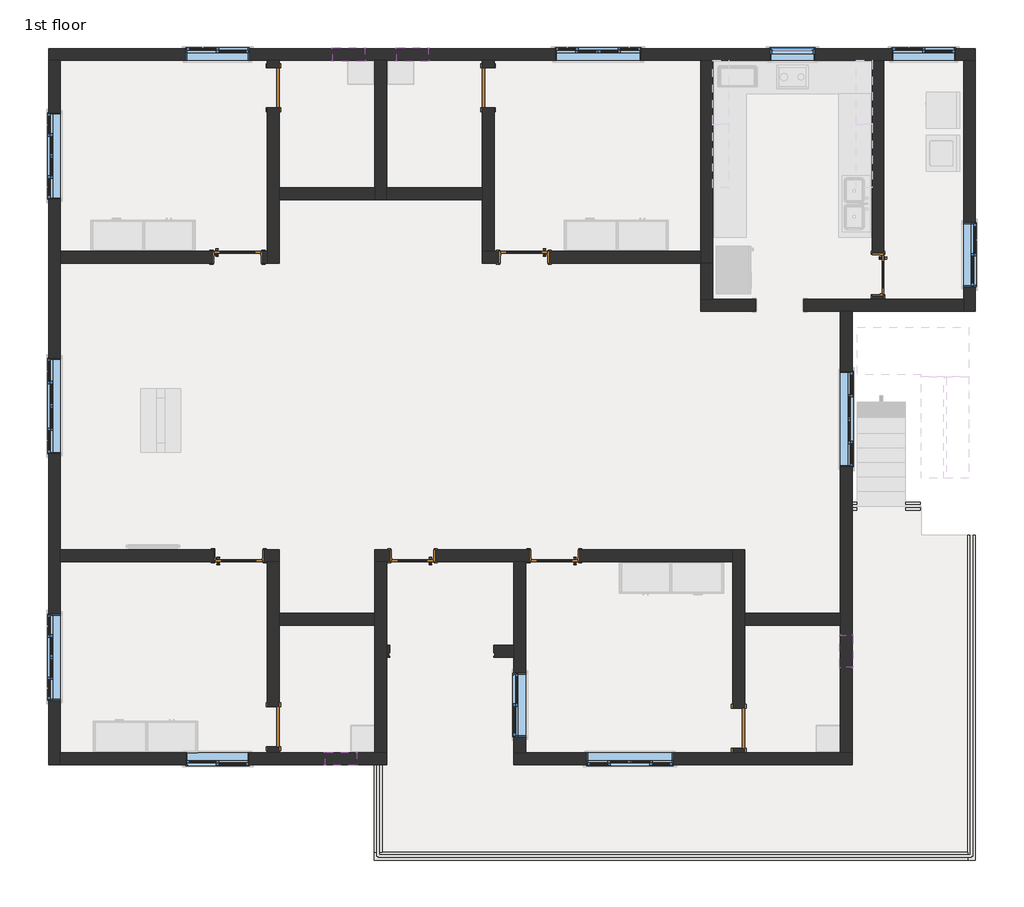
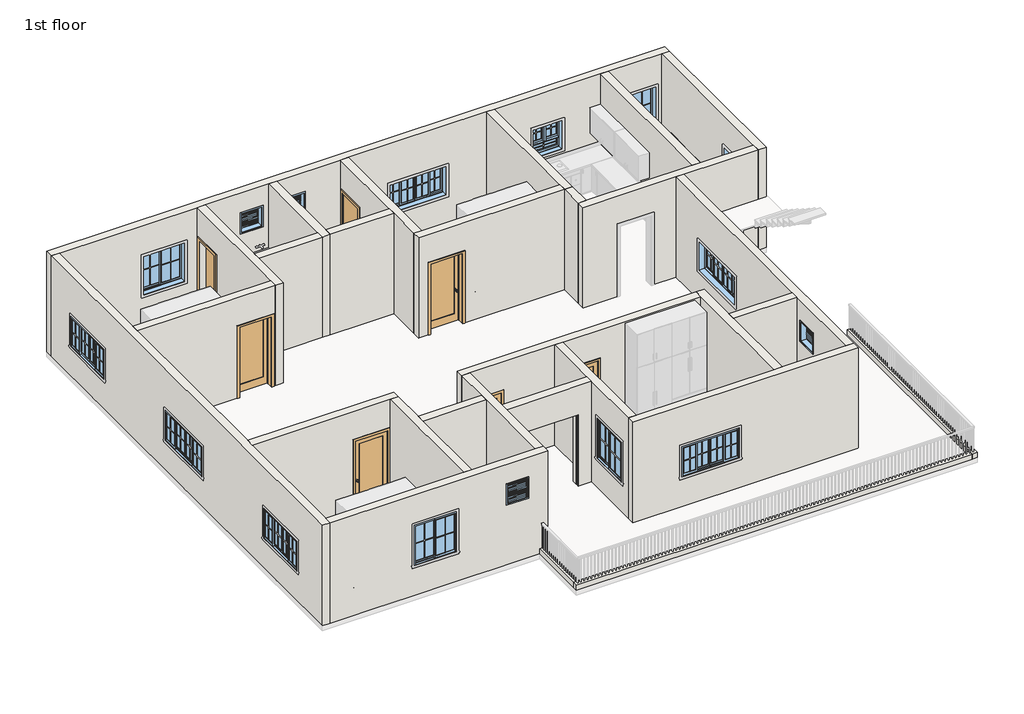
# One storey, part 1 of 4: 31 walls, 16 windows, 10 doors.
# Revit data of these elements (continued)
# Type "Window-Sliding-Four : 65\" x 36\"" (continued)
#   Interior Wall Closure [instance default] = 0' - 2 19/32"
#   Heat Transfer Coefficient (U) = 0.5511 BTU/(h·ft²·°F)
#   Frame Extension [instance default] = 0' - 0 1/4"
#   Exterior Wall Closure [instance default] = 0' - 1 1/4"
#   Rough Width = 5' - 5 1/2"
#   Rough Height = 3' - 0 1/2"
#   Height = 3' - 0"
#   Extension Jamb [instance default] = 0' - 2 3/4"
#   Default Sill Height = 3' - 0"
#   Width = 5' - 5"
#   Middle Muntin Visibility = yes
#   Interior Trim Visibility [instance default] = yes
#   Indicator Visibility [instance default] = yes
#   Exterior Trim Visibility [instance default] = yes
#   Side Muntin Visibility = yes
#   Extension Jamb Visibility [instance default] = yes
#   Interior Trim Material = Wood - Stained
#   Muntin Pattern = Muntin Pattern_2x2 : Muntin Pattern_2x2
#   Interior Trim = Trim-Window-Interior-Flat : Picture Frame
#   Interior Frame Material = Wood - Stained
#   Glass Panel Material = Glass
#   Exterior Trim Material = Clad - White
#   Exterior Trim = Trim-Window-Exterior-Flat : with Sill
#   Exterior Frame Material = Clad - White
#   Wall Closure = (empty or 0)
# Type "Window-Sliding-Four : 72\" x 36\""
#   Type Mark = "20"
#   Fire Rating = "0.5h"
#   Assembly Code = "B2020100"
#   Analytic Construction = "Double glazing - domestic"
#   Window Inset [instance default] = 0' - 0"
#   Wall Thickness [instance default] = 0' - 6"
#   Visual Light Transmittance = 0.81
#   Thermal Resistance (R) = 1.8146 (h·ft²·°F)/BTU
#   Solar Heat Gain Coefficient = 0.76
#   Interior Wall Closure [instance default] = 0' - 2 19/32"
#   Heat Transfer Coefficient (U) = 0.5511 BTU/(h·ft²·°F)
#   Frame Extension [instance default] = 0' - 0 1/4"
#   Exterior Wall Closure [instance default] = 0' - 1 1/4"
#   Rough Width = 6' - 0 1/2"
#   Rough Height = 3' - 0 1/2"
#   Height = 3' - 0"
#   Extension Jamb [instance default] = 0' - 2 3/4"
#   Default Sill Height = 3' - 0"
#   Width = 6' - 0"
#   Middle Muntin Visibility = yes
#   Interior Trim Visibility [instance default] = yes
#   Indicator Visibility [instance default] = yes
#   Exterior Trim Visibility [instance default] = yes
#   Side Muntin Visibility = yes
#   Extension Jamb Visibility [instance default] = yes
#   Interior Trim Material = Wood - Stained
#   Muntin Pattern = Muntin Pattern_2x2 : Muntin Pattern_2x2
#   Interior Trim = Trim-Window-Interior-Flat : Picture Frame
#   Interior Frame Material = Wood - Stained
#   Glass Panel Material = Glass
#   Exterior Trim Material = Clad - White
#   Exterior Trim = Trim-Window-Exterior-Flat : with Sill
#   Exterior Frame Material = Clad - White
#   Wall Closure = (empty or 0)
# Element 1 (IfcDoor, "Door-Interior-Single-1_Panel-Wood : 30\" x 84\"")
#   Swing Angle = 90.00°
#   Phase Created = New Construction
#   Materials on its faces: "Cherry", "Aluminum"
# Elements 2, 3, 4, 5 (IfcDoor, "Door-Interior-Single-1_Panel-Wood : 36\" x 84\"")
#   Swing Angle = 90.00°
#   Phase Created = New Construction
#   Materials on its faces: "Cherry", "Aluminum"
# Element 6 (IfcDoor, "Door-Interior-Single-Full Glass-Wood : 32\" x 84\"")
#   Swing Angle = 90.00°
#   Show Grill = yes
#   Phase Created = New Construction
#   Materials on its faces: "Cherry", "Aluminum", "Glass"
# Elements 7, 8, 9, 10 (IfcDoor, "Single-Flush : 30\" x 84\"")
#   Phase Created = New Construction
#   Materials on its faces: "Door - Frame", "Door - Panel"
# Elements 11, 12, 13, 14, 15 (IfcWall, "Generic - 6\"")
#   Top Offset = 0' - 0"
#   Base Offset = 0' - 0"
#   Unconnected Height = 0' - 6"
#   wall height = 0' - 6"
#   Phase Created = New Construction
#   Base Constraint = 1st floor
#   Materials on its faces: "Default Wall"
# Elements 16, 17, 18, 19, 20, 21, 22, 23, 24, 25, 26, 27, 28, 29, 30, 31, 32, 33, 34, 35, 36, 37, 38, 39, 40, 41 (IfcWall, "Generic - 9\"")
#   Top Offset = 0' - 0"
#   Base Offset = 0' - 0"
#   wall height = 10' - 0"
#   Phase Created = New Construction
#   Base Constraint = 1st floor
#   Top Constraint = 2nd floor
#   Materials on its faces: "Default Wall"
# Element 42 (IfcWindow, "Window-Casement-Double-Awning : 34\" x 36\"")
#   Mark = "38"
#   Window Inset = 0' - 0"
#   Interior Wall Closure = 0' - 2 1/4"
#   Frame Extension = 0' - 0 1/4"
#   Exterior Wall Closure = 0' - 1 1/4"
#   Interior Trim Visibility = yes
#   Exterior Trim Visibility = yes
#   Phase Created = New Construction
#   Materials on its faces: "Wood - Stained", "Glass", "Clad - White"
# Element 43 (IfcWindow, "Window-Louvers : 24\" x 24\"")
#   Mark = "32"
#   Blade Width = 1' - 10 1/2"
#   Phase Created = New Construction
#   Materials on its faces: "Birch"
# Element 44 (IfcWindow, "Window-Louvers : 24\" x 24\"")
#   Mark = "33"
#   Blade Width = 1' - 10 1/2"
#   Phase Created = New Construction
#   Materials on its faces: "Birch"
# Element 45 (IfcWindow, "Window-Louvers : 24\" x 24\"")
#   Mark = "39"
#   Blade Width = 1' - 10 1/2"
#   Phase Created = New Construction
#   Materials on its faces: "Birch"
# Element 46 (IfcWindow, "Window-Louvers : 24\" x 24\"")
#   Mark = "40"
#   Blade Width = 1' - 10 1/2"
#   Phase Created = New Construction
#   Materials on its faces: "Birch"
# Element 47 (IfcWindow, "Window-Sliding-Double : 48\" x 48\"")
#   Mark = "29"
#   Window Inset = 0' - 0"
#   Interior Wall Closure = 0' - 2 3/4"
#   Frame Extension = 0' - 0 1/4"
#   Exterior Wall Closure = 0' - 1 1/4"
#   Interior Trim Visibility = yes
#   Indicator Visibility = yes
#   Exterior Trim Visibility = yes
#   Phase Created = New Construction
#   Materials on its faces: "Wood - Stained", "Glass", "Clad - White"
# Element 48 (IfcWindow, "Window-Sliding-Double : 48\" x 48\"")
#   Mark = "30"
#   Window Inset = 0' - 0"
#   Interior Wall Closure = 0' - 2 3/4"
#   Frame Extension = 0' - 0 1/4"
#   Exterior Wall Closure = 0' - 1 1/4"
#   Interior Trim Visibility = yes
#   Indicator Visibility = yes
#   Exterior Trim Visibility = yes
#   Phase Created = New Construction
#   Materials on its faces: "Wood - Stained", "Glass", "Clad - White"
# Element 49 (IfcWindow, "Window-Sliding-Double : 48\" x 48\"")
#   Mark = "31"
#   Window Inset = 0' - 0"
#   Interior Wall Closure = 0' - 2 3/4"
#   Frame Extension = 0' - 0 1/4"
#   Exterior Wall Closure = 0' - 1 1/4"
#   Interior Trim Visibility = yes
#   Indicator Visibility = yes
#   Exterior Trim Visibility = yes
#   Phase Created = New Construction
#   Materials on its faces: "Wood - Stained", "Glass", "Clad - White"
# Element 50 (IfcWindow, "Window-Sliding-Double : 48\" x 48\"")
#   Mark = "36"
#   Window Inset = 0' - 0"
#   Interior Wall Closure = 0' - 2 3/4"
#   Frame Extension = 0' - 0 1/4"
#   Exterior Wall Closure = 0' - 1 1/4"
#   Interior Trim Visibility = yes
#   Indicator Visibility = yes
#   Exterior Trim Visibility = yes
#   Phase Created = New Construction
#   Materials on its faces: "Wood - Stained", "Glass", "Clad - White"
# Element 51 (IfcWindow, "Window-Sliding-Double : 48\" x 48\"")
#   Mark = "37"
#   Window Inset = 0' - 0"
#   Interior Wall Closure = 0' - 2 3/4"
#   Frame Extension = 0' - 0 1/4"
#   Exterior Wall Closure = 0' - 1 1/4"
#   Interior Trim Visibility = yes
#   Indicator Visibility = yes
#   Exterior Trim Visibility = yes
#   Phase Created = New Construction
#   Materials on its faces: "Wood - Stained", "Glass", "Clad - White"
# Element 52 (IfcWindow, "Window-Sliding-Four : 65\" x 36\"")
#   Mark = "25"
#   Window Inset = 0' - 0"
#   Interior Wall Closure = 0' - 2 3/4"
#   Frame Extension = 0' - 0 1/4"
#   Exterior Wall Closure = 0' - 1 1/4"
#   Interior Trim Visibility = yes
#   Indicator Visibility = yes
#   Exterior Trim Visibility = yes
#   Phase Created = New Construction
#   Materials on its faces: "Wood - Stained", "Glass", "Clad - White"
# Element 53 (IfcWindow, "Window-Sliding-Four : 65\" x 36\"")
#   Mark = "26"
#   Window Inset = 0' - 0"
#   Interior Wall Closure = 0' - 2 3/4"
#   Frame Extension = 0' - 0 1/4"
#   Exterior Wall Closure = 0' - 1 1/4"
#   Interior Trim Visibility = yes
#   Indicator Visibility = yes
#   Exterior Trim Visibility = yes
#   Phase Created = New Construction
#   Materials on its faces: "Wood - Stained", "Glass", "Clad - White"
# Element 54 (IfcWindow, "Window-Sliding-Four : 65\" x 36\"")
#   Mark = "34"
#   Window Inset = 0' - 0"
#   Interior Wall Closure = 0' - 2 3/4"
#   Frame Extension = 0' - 0 1/4"
#   Exterior Wall Closure = 0' - 1 1/4"
#   Interior Trim Visibility = yes
#   Indicator Visibility = yes
#   Exterior Trim Visibility = yes
#   Phase Created = New Construction
#   Materials on its faces: "Wood - Stained", "Glass", "Clad - White"
# Element 55 (IfcWindow, "Window-Sliding-Four : 65\" x 36\"")
#   Mark = "35"
#   Window Inset = 0' - 0"
#   Interior Wall Closure = 0' - 2 3/4"
#   Frame Extension = 0' - 0 1/4"
#   Exterior Wall Closure = 0' - 1 1/4"
#   Interior Trim Visibility = yes
#   Indicator Visibility = yes
#   Exterior Trim Visibility = yes
#   Phase Created = New Construction
#   Materials on its faces: "Wood - Stained", "Glass", "Clad - White"
# Element 56 (IfcWindow, "Window-Sliding-Four : 72\" x 36\"")
#   Mark = "27"
#   Window Inset = 0' - 0"
#   Interior Wall Closure = 0' - 2 19/32"
#   Frame Extension = 0' - 0 1/4"
#   Exterior Wall Closure = 0' - 1 1/4"
#   Interior Trim Visibility = yes
#   Indicator Visibility = yes
#   Exterior Trim Visibility = yes
#   Phase Created = New Construction
#   Materials on its faces: "Wood - Stained", "Glass", "Clad - White"
# Element 57 (IfcWindow, "Window-Sliding-Four : 72\" x 36\"")
#   Mark = "28"
#   Window Inset = 0' - 0"
#   Interior Wall Closure = 0' - 2 19/32"
#   Frame Extension = 0' - 0 1/4"
#   Exterior Wall Closure = 0' - 1 1/4"
#   Interior Trim Visibility = yes
#   Indicator Visibility = yes
#   Exterior Trim Visibility = yes
#   Phase Created = New Construction
#   Materials on its faces: "Wood - Stained", "Glass", "Clad - White"
# Materials
#   "Cherry": class "Wood", colour RGB 226 177 128, transparency 0, Description = "Prunus Serotina", Cost = 0
#   "Aluminum": class "Metal", colour RGB 247 247 247, transparency 0, Description = "Aluminum 6061", Cost = 0
#   "Door - Panel": class "Wood", colour RGB 210 159 95, transparency 0, Cost = 0
#   "Door - Frame": colour RGB 118 70 51, transparency 0, Cost = 0
#   "Wood - Stained": class "Wood", colour RGB 224 178 126, transparency 0, Cost = 0
#   "Clad - White": class "Wood", colour RGB 242 242 238, transparency 0, Cost = 0
#   "Glass": class "Glass", colour RGB 0 128 192, transparency 0.75, Description = "Soda Lime Glass", Cost = 0
#   "Birch": class "Wood", colour RGB 224 178 126, transparency 0, Description = "Betula Alleghaniensis", Cost = 0
#   "Default Wall": colour RGB 128 128 128, transparency 0, Cost = 0
